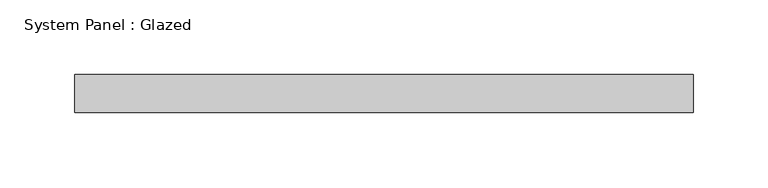
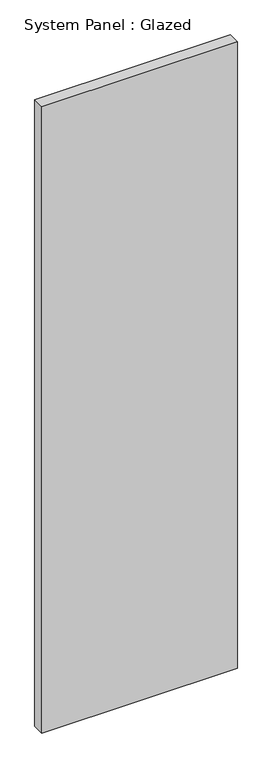
"""IFC4 building model written with IfcOpenShell, lengths in millimetres: plate geometry, System Panel : Glazed."""

from ifc_helpers import new_model, si_unit, origin, origin_with_axes, place, context, project, spatial, polyline, outline, extrude, source, transform, mapped, element, save


def system_panel_glazed_d22dc6a9(model_context):
    return source(origin(), model_context, "Body", "SweptSolid", [
        extrude(outline(polyline([(206.375, 19.05), (-206.375, 19.05), (-206.375, 44.45), (206.375, 44.45), (206.375, 19.05)])), origin_with_axes(), (0.0, 0.0, 1.0), 1397.0),
    ])


if __name__ == "__main__":
    model = new_model("IFC4")
    model_context = context("Model", 3, world=origin())
    ifc_project = project(units=[si_unit("LENGTHUNIT", "METRE", prefix="MILLI")], contexts=[model_context])
    site = spatial("IfcSite", under=ifc_project)
    building = spatial("IfcBuilding", under=site)
    placement = place(None, origin())
    system_panel_glazed_shape = system_panel_glazed_d22dc6a9(model_context)
    element("IfcPlate", 1, ObjectType="System Panel : Glazed", at=placement, inside=building, context=model_context, shape_type="MappedRepresentation", body=[
        mapped(system_panel_glazed_shape, transform((0.0, 0.0, 0.0), x_axis=(1.0, 0.0, 0.0), y_axis=(0.0, 1.0, 0.0), z_axis=(0.0, 0.0, 1.0))),
    ])
    save(model, "model.ifc")

# Revit data of these elements
# Type "System Panel : Glazed"
#   Construction Type Id = "GSP4R"
#   Analytic Construction = "1/8 in Pilkington single glazing"
#   Visual Light Transmittance = 0.9
#   Solar Heat Gain Coefficient = 0.86
#   Heat Transfer Coefficient (U) = 1.18115 BTU/(h·ft²·°F)
#   Define Thermal Properties by = 1
# Element 1 (IfcPlate, "System Panel : Glazed")
#   Materials on its faces: "Glass"
# Materials
#   "Glass": class "Glass", colour RGB 0 128 192, transparency 0.75, Description = "Soda Lime Glass", Cost = 0
